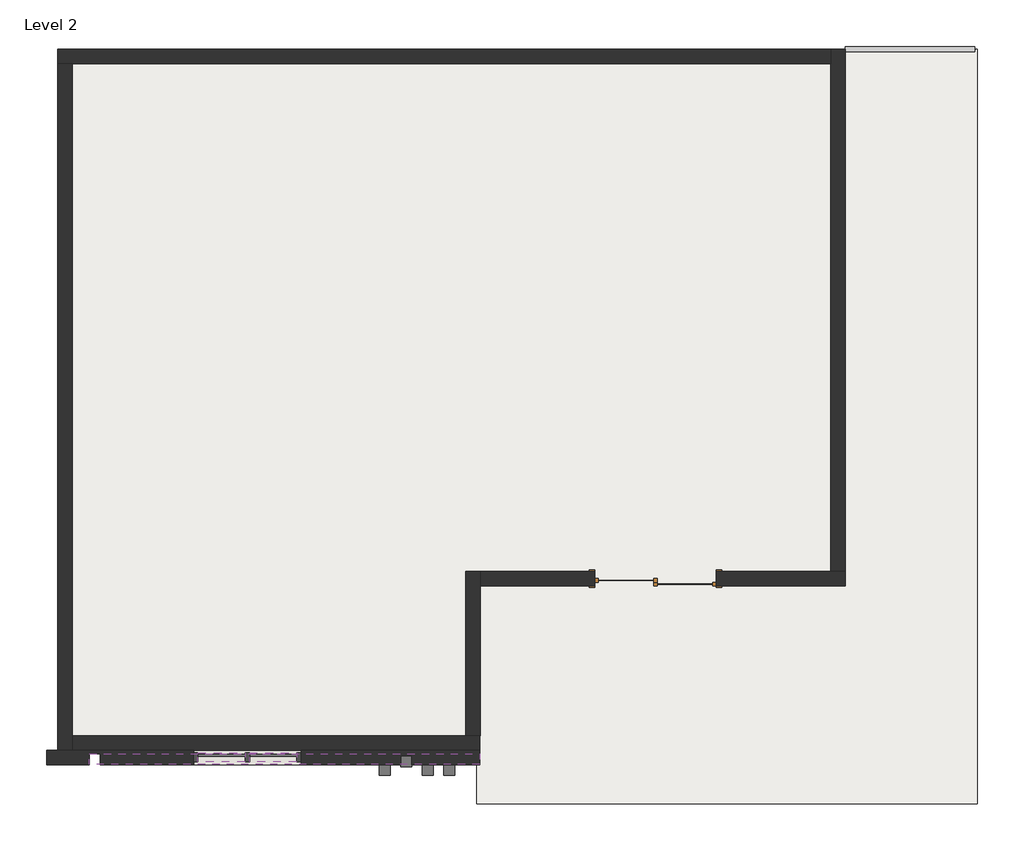
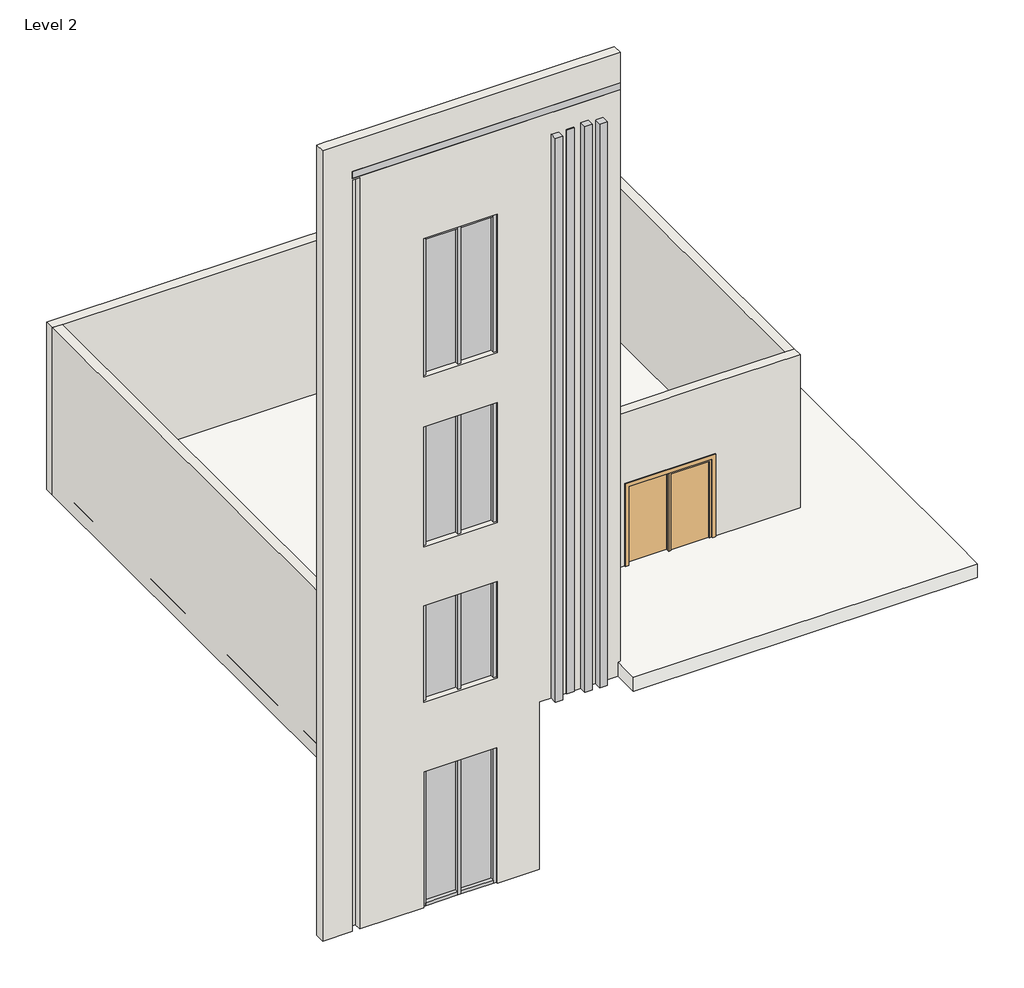
# One storey, incomplete: 7 members, 7 walls, 5 proxies, 2 plates, 1 door, 1 railing, 1 roof.
"""IFC4 building model written with IfcOpenShell, lengths in millimetres."""

from ifc_helpers import new_model, si_unit, point, frame, origin, place, context, project, spatial, polyline, ellipse_curve, trimmed, outline, extrude, faceted_brep, transform, mapped, element, save
from ifc_brep_helpers import plane_surface, extruded_surface, advanced_brep
from components import door_076b30e0, member_d41206f4, member_d26f5695, member_cf944bc0, system_panel_glazed_8086c5aa

model = new_model("IFC4")

# Units and contexts
model_context = context("Model", 3, world=origin())
ifc_project = project(units=[si_unit("LENGTHUNIT", "METRE", prefix="MILLI")], contexts=[model_context])

# Site, building, storey
site = spatial("IfcSite", under=ifc_project)
building = spatial("IfcBuilding", under=site)
storey = spatial("IfcBuildingStorey", under=building, Name="Level 2", Elevation=3657.6)

# Proxies
placement = place(None, origin())
element("IfcBuildingElementProxy", 1, Name="Cornice", ObjectType="Cornice", at=placement, inside=storey, context=model_context, shape_type="SweptSolid", body=[
    extrude(outline(polyline([(-6233.8871298, 941.3359817), (-6233.8871298, 788.9359817), (-6386.2871298, 788.9359817), (-6386.2871298, 941.3359817), (-6233.8871298, 941.3359817)])), frame((0.0, 0.0, 3657.6), z_axis=(0.0, 0.0, 1.0), x_axis=(1.0, 0.0, 0.0)), (0.0, 0.0, 1.0), 12324.0601563),
])
element("IfcBuildingElementProxy", 2, Name="Cornice", ObjectType="Cornice", at=placement, inside=storey, context=model_context, shape_type="SweptSolid", body=[
    extrude(outline(polyline([(-5929.0871298, 1064.1654287), (-5929.0871298, 911.7654287), (-6081.4871298, 911.7654287), (-6081.4871298, 1064.1654287), (-5929.0871298, 1064.1654287)])), frame((0.0, 0.0, 3657.6), z_axis=(0.0, 0.0, 1.0), x_axis=(1.0, 0.0, 0.0)), (0.0, 0.0, 1.0), 12324.0601563),
])
element("IfcBuildingElementProxy", 3, Name="Cornice", ObjectType="Cornice", at=placement, inside=storey, context=model_context, shape_type="SweptSolid", body=[
    extrude(outline(polyline([(-5624.2871298, 941.3359817), (-5624.2871298, 788.9359817), (-5776.6871298, 788.9359817), (-5776.6871298, 941.3359817), (-5624.2871298, 941.3359817)])), frame((0.0, 0.0, 3657.6), z_axis=(0.0, 0.0, 1.0), x_axis=(1.0, 0.0, 0.0)), (0.0, 0.0, 1.0), 12369.8),
])
element("IfcBuildingElementProxy", 4, Name="Cornice", ObjectType="Cornice", at=placement, inside=storey, context=model_context, shape_type="SweptSolid", body=[
    extrude(outline(polyline([(-5319.4871298, 941.3359817), (-5319.4871298, 788.9359817), (-5471.8871298, 788.9359817), (-5471.8871298, 941.3359817), (-5319.4871298, 941.3359817)])), frame((0.0, 0.0, 3657.6), z_axis=(0.0, 0.0, 1.0), x_axis=(1.0, 0.0, 0.0)), (0.0, 0.0, 1.0), 12324.0601563),
])
element("IfcBuildingElementProxy", 5, Name="Reveal", ObjectType="Reveal", at=placement, inside=storey, context=model_context, shape_type="SweptSolid", body=[
    extrude(outline(polyline([(-10501.0871298, 941.3359817), (-10501.0871298, 1093.7359817), (-4963.8871298, 1093.7359817), (-4963.8871298, 941.3359817), (-10501.0871298, 941.3359817)])), frame((0.0, 0.0, 16459.2), z_axis=(0.0, 0.0, 1.0), x_axis=(1.0, 0.0, 0.0)), (0.0, 0.0, 1.0), 152.4),
])

# Door
door_shape = door_076b30e0(model_context)
element("IfcDoor", 6, ObjectType="Door-Double-Sliding : 68\" x 80\"", at=placement, inside=storey, context=model_context, shape_type="MappedRepresentation", body=[
    mapped(door_shape, transform((-2468.3371298, 3709.9359817, 3657.6), x_axis=(-1.0, 0.0, 0.0), y_axis=(0.0, -1.0, 0.0), z_axis=(0.0, 0.0, 1.0))),
])

# Members
member_shape = member_d41206f4(model_context)
element("IfcMember", 7, ObjectType="Rectangular Mullion : 2.5\" x 5\" rectangular", at=placement, inside=storey, context=model_context, shape_type="MappedRepresentation", body=[
    mapped(member_shape, transform((-8292.8746298, 1042.9359817, 14630.4), x_axis=(0.0, 0.0, 1.0), y_axis=(0.0, -1.0, 0.0), z_axis=(1.0, 0.0, 0.0))),
])
element("IfcMember", 8, ObjectType="Rectangular Mullion : 2.5\" x 5\" rectangular", at=placement, inside=storey, context=model_context, shape_type="MappedRepresentation", body=[
    mapped(member_shape, transform((-7561.0371298, 1042.9359817, 14630.4), x_axis=(0.0, 0.0, 1.0), y_axis=(0.0, -1.0, 0.0), z_axis=(1.0, 0.0, 0.0))),
])
member_2_shape = member_d26f5695(model_context)
element("IfcMember", 9, ObjectType="Rectangular Mullion : 2.5\" x 5\" rectangular", at=placement, inside=storey, context=model_context, shape_type="MappedRepresentation", body=[
    mapped(member_2_shape, transform((-8261.1246298, 1042.9359817, 0.0), x_axis=(1.0, 0.0, 0.0), y_axis=(0.0, -1.0, 0.0), z_axis=(0.0, 0.0, -1.0))),
])
element("IfcMember", 10, ObjectType="Rectangular Mullion : 2.5\" x 5\" rectangular", at=placement, inside=storey, context=model_context, shape_type="MappedRepresentation", body=[
    mapped(member_shape, transform((-8229.3746298, 1042.9359817, 0.0), x_axis=(0.0, 0.0, -1.0), y_axis=(0.0, -1.0, 0.0), z_axis=(-1.0, 0.0, 0.0))),
])
element("IfcMember", 11, ObjectType="Rectangular Mullion : 2.5\" x 5\" rectangular", at=placement, inside=storey, context=model_context, shape_type="MappedRepresentation", body=[
    mapped(member_shape, transform((-8961.2121298, 1042.9359817, 0.0), x_axis=(0.0, 0.0, -1.0), y_axis=(0.0, -1.0, 0.0), z_axis=(-1.0, 0.0, 0.0))),
])
member_3_shape = member_cf944bc0(model_context)
element("IfcMember", 12, ObjectType="Rectangular Mullion : 2.5\" x 5\" rectangular", at=placement, inside=storey, context=model_context, shape_type="MappedRepresentation", body=[
    mapped(member_3_shape, transform((-7497.5371298, 1042.9359817, 0.0), x_axis=(1.0, 0.0, 0.0), y_axis=(0.0, -1.0, 0.0), z_axis=(0.0, 0.0, -1.0))),
])
element("IfcMember", 13, ObjectType="Rectangular Mullion : 2.5\" x 5\" rectangular", at=placement, inside=storey, context=model_context, shape_type="MappedRepresentation", body=[
    mapped(member_3_shape, transform((-9024.7121298, 1042.9359817, 14630.4), x_axis=(-1.0, 0.0, 0.0), y_axis=(0.0, -1.0, 0.0), z_axis=(0.0, 0.0, 1.0))),
])

# Plates
system_panel_glazed_shape = system_panel_glazed_8086c5aa(model_context)
element("IfcPlate", 14, ObjectType="System Panel : Glazed", at=placement, inside=storey, context=model_context, shape_type="MappedRepresentation", body=[
    mapped(system_panel_glazed_shape, transform((-8627.0433798, 1042.9359817, 63.5), x_axis=(1.0, 0.0, 0.0), y_axis=(0.0, 1.0, 0.0), z_axis=(0.0, 0.0, 1.0))),
])
element("IfcPlate", 15, ObjectType="System Panel : Glazed", at=placement, inside=storey, context=model_context, shape_type="MappedRepresentation", body=[
    mapped(system_panel_glazed_shape, transform((-7895.2058798, 1042.9359817, 63.5), x_axis=(1.0, 0.0, 0.0), y_axis=(0.0, 1.0, 0.0), z_axis=(0.0, 0.0, 1.0))),
])

# Railing
element("IfcRailing", 16, ObjectType="Glass Panel - Bottom Fill", at=placement, inside=storey, context=model_context, shape_type="SolidModel", body=[
    advanced_brep(
    [(2062.5612535, 11063.2359817, 4572.0), (2062.5612535, 11139.4359817, 4572.0), (224.0628702, 11063.2359817, 4572.0), (224.0628702, 11139.4359817, 4572.0)],
    [
        (0, 1, ellipse_curve(frame((2062.5612535, 11101.3359817, 4572.0), z_axis=(1.0, 0.0, 0.0), x_axis=(0.0, 1.0, 0.0)), 38.1, 28.575)),
        (1, 0, ellipse_curve(frame((2062.5612535, 11101.3359817, 4572.0), z_axis=(1.0, 0.0, 0.0), x_axis=(0.0, 1.0, 0.0)), 38.1, 28.575)),
        (2, 3, ellipse_curve(frame((224.0628702, 11101.3359817, 4572.0), z_axis=(-1.0, 0.0, 0.0), x_axis=(0.0, 1.0, 0.0)), 38.1, 28.575)),
        (3, 2, ellipse_curve(frame((224.0628702, 11101.3359817, 4572.0), z_axis=(-1.0, 0.0, 0.0), x_axis=(0.0, 1.0, 0.0)), 38.1, 28.575)),
        (0, 2),
        (3, 1),
    ],
    [
        plane_surface(frame((2062.5612535, 11101.3359817, 4572.0), z_axis=(1.0, 0.0, 0.0), x_axis=(0.0, -1.0, 0.0))),
        plane_surface(frame((224.0628702, 11101.3359817, 4572.0), z_axis=(-1.0, 0.0, 0.0), x_axis=(0.0, -1.0, 0.0))),
        extruded_surface(trimmed(ellipse_curve(frame((224.0628702, 11101.3359817, 4572.0), z_axis=(1.0, 0.0, 0.0), x_axis=(0.0, 1.0, 0.0)), 38.1, 28.575), [point((224.0628702, 11063.2359817, 4572.0))], [point((224.0628702, 11139.4359817, 4572.0))], True, "CARTESIAN"), (1838.4983833000001, 0.0, 0.0), 1838.4983833000001),
        extruded_surface(trimmed(ellipse_curve(frame((224.0628702, 11101.3359817, 4572.0), z_axis=(1.0, 0.0, 0.0), x_axis=(0.0, 1.0, 0.0)), 38.1, 28.575), [point((224.0628702, 11139.4359817, 4572.0))], [point((224.0628702, 11063.2359817, 4572.0))], True, "CARTESIAN"), (1838.4983833000001, 0.0, 0.0), 1838.4983833000001),
    ],
    [
        (0, [[1, 2]]),
        (1, [[3, 4]]),
        (2, [[-1, 5, -4, 6]]),
        (3, [[-2, -6, -3, -5]]),
    ],
),
    extrude(outline(polyline([(2062.5612535, 11114.0359817), (2062.5612535, 11088.6359817), (224.0628702, 11088.6359817), (224.0628702, 11114.0359817), (2062.5612535, 11114.0359817)])), frame((0.0, 0.0, 4457.7), z_axis=(0.0, 0.0, 1.0), x_axis=(1.0, 0.0, 0.0)), (0.0, 0.0, 1.0), 25.4),
    extrude(outline(polyline([(2062.5612535, 11114.0359817), (2062.5612535, 11088.6359817), (224.0628702, 11088.6359817), (224.0628702, 11114.0359817), (2062.5612535, 11114.0359817)])), frame((0.0, 0.0, 4356.1), z_axis=(0.0, 0.0, 1.0), x_axis=(1.0, 0.0, 0.0)), (0.0, 0.0, 1.0), 25.4),
    extrude(outline(polyline([(336.8620618, 11126.7359817), (336.8620618, 11075.9359817), (324.1620618, 11075.9359817), (324.1620618, 11126.7359817), (336.8620618, 11126.7359817)])), frame((0.0, 0.0, 3657.6), z_axis=(0.0, 0.0, 1.0), x_axis=(1.0, 0.0, 0.0)), (0.0, 0.0, 1.0), 885.6788223),
    extrude(outline(polyline([(1143.3120618, 11094.8008247), (330.5120618, 11094.8008247), (330.5120618, 11101.1508247), (1143.3120618, 11101.1508247), (1143.3120618, 11094.8008247)])), frame((0.0, 0.0, 3759.2), z_axis=(0.0, 0.0, 1.0), x_axis=(1.0, 0.0, 0.0)), (0.0, 0.0, 1.0), 596.9),
    extrude(outline(polyline([(1149.6620618, 11126.7359817), (1149.6620618, 11075.9359817), (1136.9620618, 11075.9359817), (1136.9620618, 11126.7359817), (1149.6620618, 11126.7359817)])), frame((0.0, 0.0, 3657.6), z_axis=(0.0, 0.0, 1.0), x_axis=(1.0, 0.0, 0.0)), (0.0, 0.0, 1.0), 885.6788223),
    extrude(outline(polyline([(1956.1120618, 11094.8008247), (1143.3120618, 11094.8008247), (1143.3120618, 11101.1508247), (1956.1120618, 11101.1508247), (1956.1120618, 11094.8008247)])), frame((0.0, 0.0, 3759.2), z_axis=(0.0, 0.0, 1.0), x_axis=(1.0, 0.0, 0.0)), (0.0, 0.0, 1.0), 596.9),
    extrude(outline(polyline([(1962.4620618, 11126.7359817), (1962.4620618, 11075.9359817), (1949.7620618, 11075.9359817), (1949.7620618, 11126.7359817), (1962.4620618, 11126.7359817)])), frame((0.0, 0.0, 3657.6), z_axis=(0.0, 0.0, 1.0), x_axis=(1.0, 0.0, 0.0)), (0.0, 0.0, 1.0), 885.6788223),
    extrude(outline(polyline([(236.7628702, 11110.8609817), (236.7628702, 11091.8109817), (217.7128702, 11091.8109817), (217.7128702, 11110.8609817), (236.7628702, 11110.8609817)])), frame((0.0, 0.0, 3657.6), z_axis=(0.0, 0.0, 1.0), x_axis=(1.0, 0.0, 0.0)), (0.0, 0.0, 1.0), 885.6788223),
    extrude(outline(polyline([(2068.9112535, 11110.8609817), (2068.9112535, 11091.8109817), (2049.8612535, 11091.8109817), (2049.8612535, 11110.8609817), (2068.9112535, 11110.8609817)])), frame((0.0, 0.0, 3657.6), z_axis=(0.0, 0.0, 1.0), x_axis=(1.0, 0.0, 0.0)), (0.0, 0.0, 1.0), 885.6788223),
])

# Roof
element("IfcRoof", 17, ObjectType="Generic - 12\"", at=placement, inside=storey, context=model_context, shape_type="SweptSolid", body=[
    extrude(outline(polyline([(-10951.9371298, 11101.3359817), (2101.2415497, 11101.3359817), (2101.2415497, 1144.5359817), (2101.2415497, 382.5359817), (-5008.3371298, 382.5359817), (-5008.3371298, 1144.5359817), (-10951.9371298, 1144.5359817), (-10951.9371298, 11101.3359817)])), frame((0.0, 0.0, 3657.6), z_axis=(0.0, 0.0, 1.0), x_axis=(1.0, 0.0, 0.0)), (0.0, 0.0, 1.0), 304.8),
])

# Walls
element("IfcWall", 18, ObjectType="Generic - 8\"", at=placement, inside=storey, context=model_context, shape_type="Brep", body=[
    faceted_brep([(-10951.9371298, 10898.1359817, 3657.6), (-10748.7371298, 10898.1359817, 3657.6), (20.8628702, 10898.1359817, 3657.6), (20.8628702, 10898.1359817, 7315.2), (-10748.7371298, 10898.1359817, 7315.2), (-10951.9371298, 10898.1359817, 7315.2), (-10951.9371298, 11101.3359817, 3657.6), (-10951.9371298, 11101.3359817, 7315.2), (20.8628702, 11101.3359817, 7315.2), (20.8628702, 11101.3359817, 3657.6)], [[[0, 1, 2, 3, 4, 5]], [[6, 7, 8, 9]], [[2, 1, 0, 6, 9]], [[5, 4, 3, 8, 7]], [[0, 5, 7, 6]], [[3, 2, 9, 8]]]),
])
element("IfcWall", 19, ObjectType="Generic - 8\"", at=placement, inside=storey, context=model_context, shape_type="Brep", body=[
    faceted_brep([(-10748.7371298, 1144.5359817, 3657.6), (-10748.7371298, 1347.7359817, 3657.6), (-10748.7371298, 10898.1359817, 3657.6), (-10748.7371298, 10898.1359817, 7315.2), (-10748.7371298, 1347.7359817, 7315.2), (-10748.7371298, 1144.5359817, 7315.2), (-10951.9371298, 1144.5359817, 3657.6), (-10951.9371298, 1144.5359817, 7315.2), (-10951.9371298, 10898.1359817, 7315.2), (-10951.9371298, 10898.1359817, 3657.6)], [[[0, 1, 2, 3, 4, 5]], [[6, 7, 8, 9]], [[2, 1, 0, 6, 9]], [[5, 4, 3, 8, 7]], [[0, 5, 7, 6]], [[3, 2, 9, 8]]]),
])
element("IfcWall", 20, ObjectType="Generic - 8\"", at=placement, inside=storey, context=model_context, shape_type="SweptSolid", body=[
    extrude(outline(polyline([(-10748.7371298, 1347.7359817), (-4963.8871298, 1347.7359817), (-4963.8871298, 1144.5359817), (-10748.7371298, 1144.5359817), (-10748.7371298, 1347.7359817)])), frame((0.0, 0.0, 3657.6), z_axis=(0.0, 0.0, 1.0), x_axis=(1.0, 0.0, 0.0)), (0.0, 0.0, 1.0), 3657.6),
])
element("IfcWall", 21, ObjectType="Generic - 8\"", at=placement, inside=storey, context=model_context, shape_type="Brep", body=[
    faceted_brep([(20.8628702, 11101.3359817, 3657.6), (20.8628702, 10898.1359817, 3657.6), (20.8628702, 3684.5359817, 3657.6), (20.8628702, 3684.5359817, 7315.2), (20.8628702, 10898.1359817, 7315.2), (20.8628702, 11101.3359817, 7315.2), (224.0628702, 11101.3359817, 3657.6), (224.0628702, 11101.3359817, 7315.2), (224.0628702, 3684.5359817, 7315.2), (224.0628702, 3684.5359817, 3657.6)], [[[0, 1, 2, 3, 4, 5]], [[6, 7, 8, 9]], [[2, 1, 0, 6, 9]], [[5, 4, 3, 8, 7]], [[0, 5, 7, 6]], [[3, 2, 9, 8]]]),
])
element("IfcWall", 22, ObjectType="Generic - 8\"", at=placement, inside=storey, context=model_context, shape_type="Brep", body=[
    faceted_brep([(-4963.8871298, 941.3359817, 17282.1203125), (-11110.6871298, 941.3359817, 17282.1203125), (-11110.6871298, 941.3359817, 0.0), (-10501.0871298, 941.3359817, 0.0), (-10501.0871298, 941.3359817, 16422.5278597), (-10348.6871298, 941.3359817, 16422.5278597), (-10348.6871298, 941.3359817, 0.0), (-9024.7121298, 941.3359817, 0.0), (-9024.7121298, 941.3359817, 2966.9543228), (-7497.5371298, 941.3359817, 2966.9543228), (-7497.5371298, 941.3359817, 0.0), (-6633.9371298, 941.3359817, 0.0), (-6633.9371298, 941.3359817, 3657.6), (-6081.4871298, 941.3359817, 3657.6), (-6081.4871298, 941.3359817, 15981.6601563), (-5929.0871298, 941.3359817, 15981.6601563), (-5929.0871298, 941.3359817, 3657.6), (-4963.8871298, 941.3359817, 3657.6), (-4963.8871298, 941.3359817, 16459.2), (-10501.0871298, 941.3359817, 16459.2), (-10501.0871298, 941.3359817, 16611.6), (-4963.8871298, 941.3359817, 16611.6), (-7497.5371298, 941.3359817, 14630.4), (-7497.5371298, 941.3359817, 11600.7604649), (-9024.7121298, 941.3359817, 11600.7604649), (-9024.7121298, 941.3359817, 14630.4), (-7497.5371298, 941.3359817, 10503.1578883), (-7497.5371298, 941.3359817, 7885.8823571), (-9024.7121298, 941.3359817, 7885.8823571), (-9024.7121298, 941.3359817, 10503.1578883), (-7497.5371298, 941.3359817, 6594.5866784), (-7497.5371298, 941.3359817, 4490.9543228), (-9024.7121298, 941.3359817, 4490.9543228), (-9024.7121298, 941.3359817, 6594.5866784), (-4963.8871298, 1144.5359817, 17282.1203125), (-4963.8871298, 1144.5359817, 3657.6), (-6633.9371298, 1144.5359817, 3657.6), (-6633.9371298, 1144.5359817, 0.0), (-7497.5371298, 1144.5359817, 0.0), (-7497.5371298, 1144.5359817, 2966.9543228), (-9024.7121298, 1144.5359817, 2966.9543228), (-9024.7121298, 1144.5359817, 0.0), (-11110.6871298, 1144.5359817, 0.0), (-11110.6871298, 1144.5359817, 17282.1203125), (-10951.9371298, 1144.5359817, 17282.1203125), (-10748.7371298, 1144.5359817, 17282.1203125), (-7497.5371298, 1144.5359817, 11600.7604649), (-7497.5371298, 1144.5359817, 14630.4), (-9024.7121298, 1144.5359817, 14630.4), (-9024.7121298, 1144.5359817, 11600.7604649), (-7497.5371298, 1144.5359817, 7885.8823571), (-7497.5371298, 1144.5359817, 10503.1578883), (-9024.7121298, 1144.5359817, 10503.1578883), (-9024.7121298, 1144.5359817, 7885.8823571), (-7497.5371298, 1144.5359817, 4490.9543228), (-7497.5371298, 1144.5359817, 6594.5866784), (-9024.7121298, 1144.5359817, 6594.5866784), (-9024.7121298, 1144.5359817, 4490.9543228), (-4963.8871298, 1093.7359817, 16611.6), (-4963.8871298, 1093.7359817, 16459.2), (-5929.0871298, 1064.1654287, 3657.6), (-6081.4871298, 1064.1654287, 3657.6), (-10348.6871298, 1093.7359817, 0.0), (-10501.0871298, 1093.7359817, 0.0), (-10501.0871298, 1093.7359817, 16422.5278597), (-10348.6871298, 1093.7359817, 16422.5278597), (-10501.0871298, 1093.7359817, 16611.6), (-10501.0871298, 1093.7359817, 16459.2), (-6081.4871298, 1064.1654287, 15981.6601563), (-5929.0871298, 1064.1654287, 15981.6601563)], [[[0, 1, 2, 3, 4, 5, 6, 7, 8, 9, 10, 11, 12, 13, 14, 15, 16, 17, 18, 19, 20, 21], [22, 23, 24, 25], [26, 27, 28, 29], [30, 31, 32, 33]], [[34, 35, 36, 37, 38, 39, 40, 41, 42, 43, 44, 45], [46, 47, 48, 49], [50, 51, 52, 53], [54, 55, 56, 57]], [[35, 34, 0, 21, 58, 59, 18, 17]], [[1, 0, 34, 45, 44, 43]], [[2, 1, 43, 42]], [[12, 11, 37, 36]], [[36, 35, 17, 16, 60, 61, 13, 12]], [[42, 41, 7, 6, 62, 63, 3, 2]], [[8, 7, 41, 40]], [[9, 8, 40, 39]], [[10, 9, 39, 38]], [[11, 10, 38, 37]], [[23, 22, 47, 46]], [[24, 23, 46, 49]], [[25, 24, 49, 48]], [[22, 25, 48, 47]], [[27, 26, 51, 50]], [[28, 27, 50, 53]], [[29, 28, 53, 52]], [[26, 29, 52, 51]], [[31, 30, 55, 54]], [[32, 31, 54, 57]], [[33, 32, 57, 56]], [[30, 33, 56, 55]], [[64, 65, 5, 4]], [[65, 62, 6, 5]], [[65, 64, 63, 62]], [[63, 64, 4, 3]], [[66, 20, 19, 67]], [[20, 66, 58, 21]], [[66, 67, 59, 58]], [[67, 19, 18, 59]], [[68, 69, 15, 14]], [[69, 68, 61, 60]], [[61, 68, 14, 13]], [[69, 60, 16, 15]]]),
])
element("IfcWall", 23, ObjectType="Generic - 8\"", at=placement, inside=storey, context=model_context, shape_type="Brep", body=[
    faceted_brep([(-4957.5371298, 1347.7359817, 3657.6), (-4957.5371298, 3481.3359817, 3657.6), (-4957.5371298, 3684.5359817, 3657.6), (-4957.5371298, 3684.5359817, 7315.2), (-4957.5371298, 3684.5359817, 9753.6), (-4957.5371298, 1347.7359817, 9753.6), (-4957.5371298, 1347.7359817, 7315.2), (-5160.7371298, 1347.7359817, 3657.6), (-5160.7371298, 1347.7359817, 9753.6), (-5160.7371298, 3684.5359817, 9753.6), (-5160.7371298, 3684.5359817, 3657.6)], [[[0, 1, 2, 3, 4, 5, 6]], [[7, 8, 9, 10]], [[2, 1, 0, 7, 10]], [[5, 4, 9, 8]], [[2, 10, 9, 4, 3]], [[0, 6, 5, 8, 7]]]),
])
element("IfcWall", 24, ObjectType="Generic - 8\"", at=placement, inside=storey, context=model_context, shape_type="Brep", body=[
    faceted_brep([(-4957.5371298, 3481.3359817, 3657.6), (-3331.9371298, 3481.3359817, 3657.6), (-3331.9371298, 3481.3359817, 5689.6), (-1604.7371298, 3481.3359817, 5689.6), (-1604.7371298, 3481.3359817, 3657.6), (224.0628702, 3481.3359817, 3657.6), (224.0628702, 3481.3359817, 7315.2), (-1604.7371298, 3481.3359817, 7315.2), (-3331.9371298, 3481.3359817, 7315.2), (-4957.5371298, 3481.3359817, 7315.2), (-3331.9371298, 3684.5359817, 5689.6), (-3331.9371298, 3684.5359817, 3657.6), (-4957.5371298, 3684.5359817, 3657.6), (-4957.5371298, 3684.5359817, 7315.2), (-3331.9371298, 3684.5359817, 7315.2), (-1604.7371298, 3684.5359817, 7315.2), (20.8628702, 3684.5359817, 7315.2), (224.0628702, 3684.5359817, 7315.2), (224.0628702, 3684.5359817, 3657.6), (20.8628702, 3684.5359817, 3657.6), (-1604.7371298, 3684.5359817, 3657.6), (-1604.7371298, 3684.5359817, 5689.6)], [[[0, 1, 2, 3, 4, 5, 6, 7, 8, 9]], [[10, 11, 12, 13, 14, 15, 16, 17, 18, 19, 20, 21]], [[12, 11, 1, 0]], [[20, 19, 18, 5, 4]], [[9, 8, 7, 6, 17, 16, 15, 14, 13]], [[0, 9, 13, 12]], [[6, 5, 18, 17]], [[4, 3, 21, 20]], [[2, 1, 11, 10]], [[3, 2, 10, 21]]]),
])

save(model, "model.ifc")

# Revit data of these elements
# Type "Door-Double-Sliding : 68\" x 80\""
#   Type Mark = "9"
#   Construction Type Id = "opn-d45"
#   Assembly Code = "C1020"
#   Analytic Construction = "Wood frame, double glass door "
#   Thickness = 0' - 2"
#   Thermal Resistance (R) = 1.8150 (h·ft²·°F)/BTU
#   Heat Transfer Coefficient (U) = 0.5510 BTU/(h·ft²·°F)
#   Height = 6' - 8"
#   Rail Width = 0' - 2"
#   Stiles = 0' - 2"
#   Trim Projection Ext = 0' - 1"
#   Trim Projection Int = 0' - 1"
#   Trim Width = 0' - 3"
#   Width = 5' - 8"
#   Define Thermal Properties by = 1
#   Glazing = Glass
#   Panel Material = Wood - Birch - Solid Stained Light Low Gloss
#   Trim Material = Paint - Sienna
#   Visual Light Transmittance = 0
#   Solar Heat Gain Coefficient = 0
#   Function = (empty or 0)
#   Wall Closure = (empty or 0)
# Type "Rectangular Mullion : 2.5\" x 5\" rectangular"
#   built-in parameter 1007304 = 0.416667 (stored number, unit not read)
#   built-in parameter 1007301 = 0.104167 (stored number, unit not read)
#   built-in parameter 1007300 = 0.104167 (stored number, unit not read)
# Type "System Panel : Glazed"
#   Construction Type Id = "GSP4R"
#   Analytic Construction = "1/8 in Pilkington single glazing"
#   Visual Light Transmittance = 0.9
#   Solar Heat Gain Coefficient = 0.86
#   Heat Transfer Coefficient (U) = 1.18115 BTU/(h·ft²·°F)
# Type "Glass Panel - Bottom Fill"
#   Assembly Code = "C2010400"
#   built-in parameter 1008612 = 0.0416667 (stored number, unit not read)
#   built-in parameter 1008611 = 0.0416667 (stored number, unit not read)
#   built-in parameter 1008609 = 0.333333 (stored number, unit not read)
#   built-in parameter 1008604 = 0.166667 (stored number, unit not read)
#   built-in parameter 1008603 = 0.166667 (stored number, unit not read)
#   Railing Height = 3' - 0"
#   built-in parameter 1008630 = 2
#   built-in parameter 1008610 = 2
#   built-in parameter 1008618 = Baluster - Square : 3/4"
# Type "Generic - 12\""
#   Assembly Code = "B1020"
#   Layers, outside or top first: 1' - 0" no material (function 1)
# Type "Generic - 8\""
#   Assembly Code = "B2010"
#   Layers, outside or top first: 0' - 8" no material (function 1)
# Elements 1, 2, 3, 4 (IfcBuildingElementProxy, "Cornice")
#   Phase Created = New Construction
#   Materials on its faces: "Default Wall"
# Element 6 (IfcDoor, "Door-Double-Sliding : 68\" x 80\"")
#   Phase Created = New Construction
#   Materials on its faces: "Paint - Sienna", "Wood - Birch - Solid Stained Light Low Gloss", "Glass"
# Elements 7, 8, 9, 10, 11, 12, 13 (IfcMember, "Rectangular Mullion : 2.5\" x 5\" rectangular")
#   Phase Created = New Construction
#   Materials on its faces: "Aluminum"
# Elements 14, 15 (IfcPlate, "System Panel : Glazed")
#   Phase Created = New Construction
#   Materials on its faces: "Glass"
# Element 16 (IfcRailing, "Glass Panel - Bottom Fill")
#   Phase Created = New Construction
#   Materials on its faces: "Glass"
# Element 17 (IfcRoof, "Generic - 12\"")
#   built-in parameter 1001705 = 13 (stored number, unit not read)
#   built-in parameter 1001710 = 33615
#   Phase Created = New Construction
#   Materials on its faces: "Default Roof"
# Elements 18, 19, 20, 21, 24 (IfcWall, "Generic - 8\"")
#   Top Offset = 0' - 0"
#   Base Offset = 0' - 0"
#   Unconnected Height = 12' - 0"
#   wall height = 12' - 0"
#   Phase Created = New Construction
#   Base Constraint = Level 2
#   Materials on its faces: "Default Wall"
# Element 22 (IfcWall, "Generic - 8\"")
#   built-in parameter 1001111 = -12' - 0"
#   Top Offset = 0' - 0"
#   Base Offset = -12' - 0"
#   Unconnected Height = 56' - 8 51/128"
#   wall height = 56' - 8 51/128"
#   Phase Created = New Construction
#   Base Constraint = Level 2
#   Materials on its faces: "Default Wall"
# Element 23 (IfcWall, "Generic - 8\"")
#   Top Offset = 0' - 0"
#   Base Offset = 0' - 0"
#   Unconnected Height = 20' - 0"
#   wall height = 20' - 0"
#   Phase Created = New Construction
#   Base Constraint = Level 2
#   Materials on its faces: "Default Wall"
# Materials
#   "Glass": class "Glass", colour RGB 0 128 192, transparency 0.75, Description = "Soda Lime Glass", Cost = 0
#   "Wood - Birch - Solid Stained Light Low Gloss": class "Wood", colour RGB 210 159 95, transparency 0, Cost = 0
#   "Paint - Sienna": colour RGB 118 70 51, transparency 0, Cost = 0
#   "Default Wall": colour RGB 128 128 128, transparency 0
#   "Aluminum": class "Metal", colour RGB 247 247 247, transparency 0, Description = "Aluminum 6061", Cost = 0
#   "Default Roof": colour RGB 88 101 114, transparency 0
